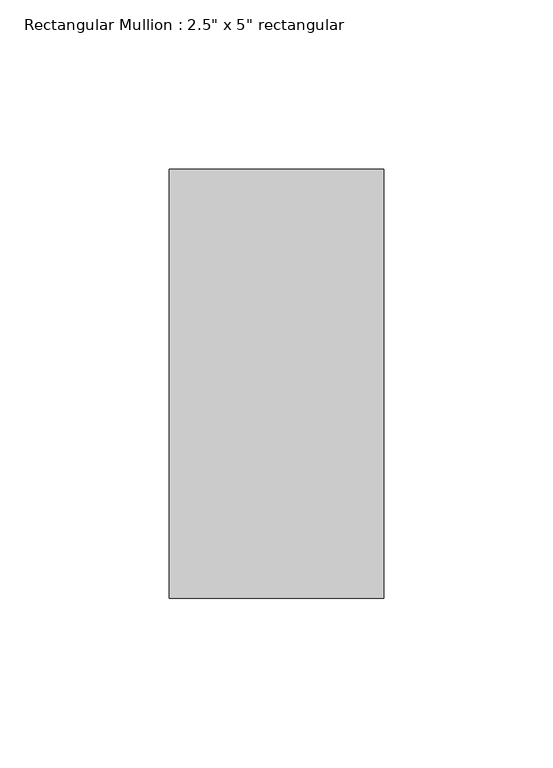
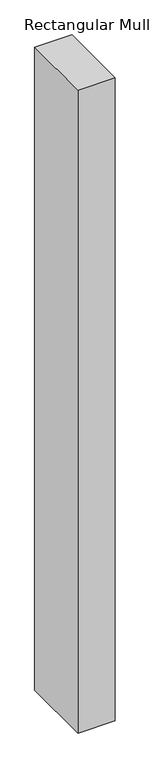
"""IFC4 building model written with IfcOpenShell, lengths in millimetres: member geometry."""

from ifc_helpers import new_model, si_unit, frame, origin, place, context, project, spatial, polyline, outline, extrude, source, transform, mapped, element, save


def member_0585f7b2(model_context):
    return source(origin(), model_context, "Body", "SweptSolid", [
        extrude(outline(polyline([(31.75, 63.5), (31.75, -63.5), (-31.75, -63.5), (-31.75, 63.5), (31.75, 63.5)])), frame((0.0, 0.0, -1155.7), z_axis=(0.0, 0.0, 1.0), x_axis=(1.0, 0.0, 0.0)), (0.0, 0.0, 1.0), 1155.7),
    ])


if __name__ == "__main__":
    model = new_model("IFC4")
    model_context = context("Model", 3, world=origin())
    ifc_project = project(units=[si_unit("LENGTHUNIT", "METRE", prefix="MILLI")], contexts=[model_context])
    site = spatial("IfcSite", under=ifc_project)
    building = spatial("IfcBuilding", under=site)
    placement = place(None, origin())
    member_shape = member_0585f7b2(model_context)
    element("IfcMember", 1, ObjectType="Rectangular Mullion : 2.5\" x 5\" rectangular", at=placement, inside=building, context=model_context, shape_type="MappedRepresentation", body=[
        mapped(member_shape, transform((0.0, 0.0, 0.0), x_axis=(1.0, 0.0, 0.0), y_axis=(0.0, 1.0, 0.0), z_axis=(0.0, 0.0, 1.0))),
    ])
    save(model, "model.ifc")

# Revit data of these elements
# Type "Rectangular Mullion : 2.5\" x 5\" rectangular"
#   built-in parameter 1007304 = 0.416667 (stored number, unit not read)
#   built-in parameter 1007301 = 0.104167 (stored number, unit not read)
#   built-in parameter 1007300 = 0.104167 (stored number, unit not read)
# Element 1 (IfcMember, "Rectangular Mullion : 2.5\" x 5\" rectangular")
#   Materials on its faces: "Aluminum"
# Materials
#   "Aluminum": class "Metal", colour RGB 247 247 247, transparency 0, Description = "Aluminum 6061", Cost = 0
